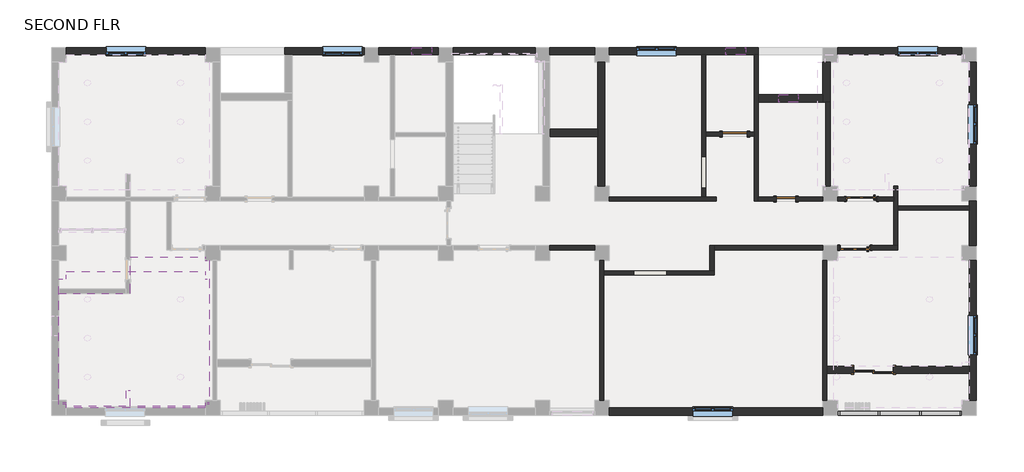
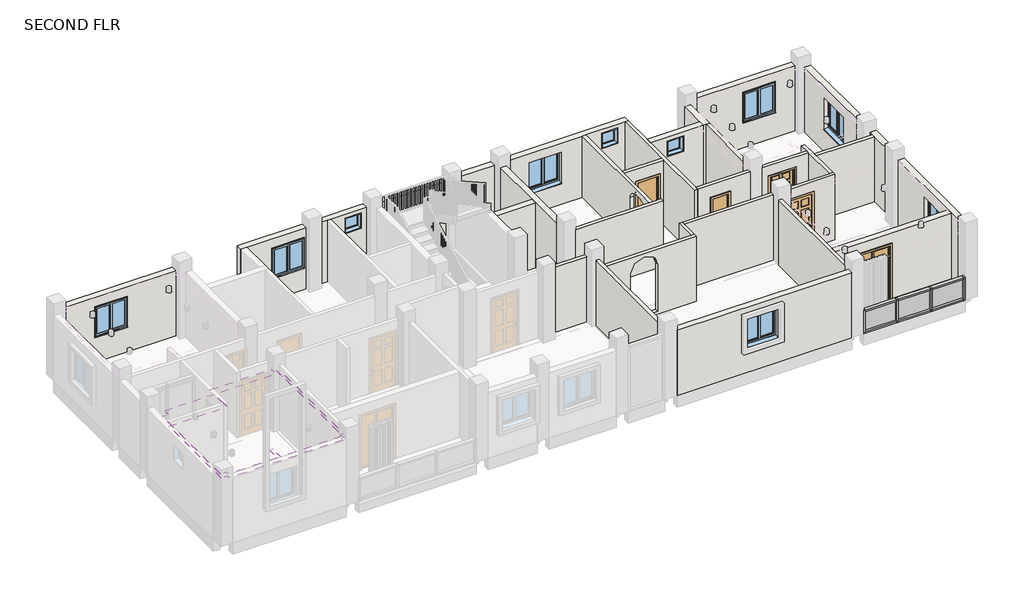
# One storey, part 2 of 5: 32 walls, 10 members, 10 windows, 5 doors, 3 plates, 2 coverings.
"""IFC4 building model written with IfcOpenShell, lengths in millimetres."""

from ifc_helpers import new_model, si_unit, point, frame, frame_2d, origin, place, context, project, spatial, polyline, circle_curve, ellipse_curve, trimmed, segment, composite_curve, outline, extrude, faceted_brep, transform, mapped, element, save
from ifc_brep_helpers import plane_surface, extruded_surface, advanced_brep
from components import door_double_sliding_4436dcad, door_c610b25b, door_03e3dfb5, single_flush_2_x_7_bath_room_door_025d1c86, door_1fe7f57d, member_5d96a33e, member_91edd790, member_410c6227, member_73c23c35, system_panel_glazed_2f542010, system_panel_glazed_876b4d55, window_80340324, w2_0001_4_x_4_window_9dec5fc7

model = new_model("IFC4")

# Units and contexts
model_context = context("Model", 3, world=origin())
ifc_project = project(units=[si_unit("LENGTHUNIT", "METRE", prefix="MILLI")], contexts=[model_context])

# Site, building, storey
site = spatial("IfcSite", under=ifc_project)
building = spatial("IfcBuilding", under=site)
storey = spatial("IfcBuildingStorey", under=building, Name="SECOND FLR", Elevation=6400.8)

# Coverings
placement = place(None, origin())
element("IfcCovering", 1, ObjectType="GWB on Mtl. Stud", at=placement, inside=storey, context=model_context, shape_type="SweptSolid", body=[
    extrude(outline(polyline([(-15145.3456086, -10773.5679047), (-15145.3456086, -7363.1659448), (-12959.7401855, -7363.1659448), (-12959.7401855, -6244.0794704), (-10649.5456086, -6244.0794704), (-10649.5456086, -6358.3794704), (-10535.2456086, -6358.3794704), (-10535.2456086, -6963.5679047), (-10535.2456086, -10773.5679047), (-10649.5456086, -10773.5679047), (-10649.5456086, -10887.8679047), (-12959.7401855, -10887.8679047), (-14916.7456086, -10887.8679047), (-14916.7456086, -10773.5679047), (-15145.3456086, -10773.5679047)]), holes=[polyline([(-14840.5456086, -10583.0679047), (-10840.0456086, -10583.0679047), (-10840.0456086, -6548.8794704), (-12654.9401855, -6548.8794704), (-12654.9401855, -7667.9659448), (-14840.5456086, -7667.9659448), (-14840.5456086, -10583.0679047)])]), frame((0.0, 0.0, 8839.2), z_axis=(0.0, 0.0, 1.0), x_axis=(1.0, 0.0, 0.0)), (0.0, 0.0, 1.0), 107.95),
    extrude(outline(polyline([(-14688.1456086, -10430.6679047), (-14688.1456086, -7820.3659448), (-12502.5401855, -7820.3659448), (-12502.5401855, -6701.2794704), (-10992.4456086, -6701.2794704), (-10992.4456086, -10430.6679047), (-14688.1456086, -10430.6679047)]), holes=[polyline([(-14535.7456086, -7972.7659448), (-14535.7456086, -10278.2679047), (-11144.8456086, -10278.2679047), (-11144.8456086, -6853.6794704), (-12350.1401855, -6853.6794704), (-12350.1401855, -7972.7659448), (-14535.7456086, -7972.7659448)])]), frame((0.0, 0.0, 8839.2), z_axis=(0.0, 0.0, 1.0), x_axis=(1.0, 0.0, 0.0)), (0.0, 0.0, 1.0), 107.95),
])
element("IfcCovering", 2, ObjectType="GWB on Mtl. Stud", at=placement, inside=storey, context=model_context, shape_type="SweptSolid", body=[
    extrude(outline(polyline([(-14916.7456086, -6917.1794704), (-14916.7456086, -6688.5794704), (-10649.5456086, -6688.5794704), (-10649.5456086, -6917.1794704), (-10535.2456086, -6917.1794704), (-10535.2456086, -10727.1794704), (-10649.5456086, -10727.1794704), (-10649.5456086, -10841.4794704), (-12959.7401855, -10841.4794704), (-12959.7401855, -10360.3659448), (-13086.7401855, -10360.3659448), (-13086.7401855, -10841.4794704), (-14916.7456086, -10841.4794704), (-14916.7456086, -10727.1794704), (-15145.3456086, -10727.1794704), (-15145.3456086, -6917.1794704), (-14916.7456086, -6917.1794704)]), holes=[composite_curve([segment(trimmed(circle_curve(frame_2d((-14269.0456086, -7552.1794704)), 76.2), [point((-14345.2456086, -7552.1794704))], [point((-14192.8456086, -7552.1794704))], True, "CARTESIAN"), True, "CONTINUOUS"), segment(trimmed(circle_curve(frame_2d((-14269.0456086, -7552.1794704)), 76.2), [point((-14192.8456086, -7552.1794704))], [point((-14345.2456086, -7552.1794704))], True, "CARTESIAN"), True, "CONTINUOUS")], self_intersect=False), composite_curve([segment(trimmed(circle_curve(frame_2d((-14269.0456086, -9939.7794704)), 76.2), [point((-14345.2456086, -9939.7794704))], [point((-14192.8456086, -9939.7794704))], True, "CARTESIAN"), True, "CONTINUOUS"), segment(trimmed(circle_curve(frame_2d((-14269.0456086, -9939.7794704)), 76.2), [point((-14192.8456086, -9939.7794704))], [point((-14345.2456086, -9939.7794704))], True, "CARTESIAN"), True, "CONTINUOUS")], self_intersect=False), composite_curve([segment(trimmed(circle_curve(frame_2d((-14269.0456086, -8745.9794704)), 76.2), [point((-14345.2456086, -8745.9794704))], [point((-14192.8456086, -8745.9794704))], True, "CARTESIAN"), True, "CONTINUOUS"), segment(trimmed(circle_curve(frame_2d((-14269.0456086, -8745.9794704)), 76.2), [point((-14192.8456086, -8745.9794704))], [point((-14345.2456086, -8745.9794704))], True, "CARTESIAN"), True, "CONTINUOUS")], self_intersect=False), composite_curve([segment(trimmed(circle_curve(frame_2d((-11411.5456086, -7552.1794704)), 76.2), [point((-11335.3456086, -7552.1794704))], [point((-11487.7456086, -7552.1794704))], True, "CARTESIAN"), True, "CONTINUOUS"), segment(trimmed(circle_curve(frame_2d((-11411.5456086, -7552.1794704)), 76.2), [point((-11487.7456086, -7552.1794704))], [point((-11335.3456086, -7552.1794704))], True, "CARTESIAN"), True, "CONTINUOUS")], self_intersect=False), composite_curve([segment(trimmed(circle_curve(frame_2d((-11411.5456086, -9939.7794704)), 76.2), [point((-11335.3456086, -9939.7794704))], [point((-11487.7456086, -9939.7794704))], True, "CARTESIAN"), True, "CONTINUOUS"), segment(trimmed(circle_curve(frame_2d((-11411.5456086, -9939.7794704)), 76.2), [point((-11487.7456086, -9939.7794704))], [point((-11335.3456086, -9939.7794704))], True, "CARTESIAN"), True, "CONTINUOUS")], self_intersect=False)]), frame((0.0, 0.0, 8966.2), z_axis=(0.0, 0.0, 1.0), x_axis=(1.0, 0.0, 0.0)), (0.0, 0.0, 1.0), 107.95),
])

# Doors
door_double_sliding_shape = door_double_sliding_4436dcad(model_context)
element("IfcDoor", 3, ObjectType="Door-Double-Sliding", at=placement, inside=storey, context=model_context, shape_type="MappedRepresentation", body=[
    mapped(door_double_sliding_shape, transform((9879.3128058, -9592.4679047, 6400.8), x_axis=(-1.0, 0.0, 0.0), y_axis=(0.0, -1.0, 0.0), z_axis=(0.0, 0.0, 1.0))),
])
door_shape = door_c610b25b(model_context)
element("IfcDoor", 4, ObjectType="Door-Interior-Single-6_Panel-Wood : 36\" x 84\"", at=placement, inside=storey, context=model_context, shape_type="MappedRepresentation", body=[
    mapped(door_shape, transform((9511.0128058, -4462.9044704, 6400.8), x_axis=(-1.0, 0.0, 0.0), y_axis=(0.0, -1.0, 0.0), z_axis=(0.0, 0.0, 1.0))),
])
door_2_shape = door_03e3dfb5(model_context)
element("IfcDoor", 5, ObjectType="Door-Interior-Single-6_Panel-Wood : 36\" x 84\"", at=placement, inside=storey, context=model_context, shape_type="MappedRepresentation", body=[
    mapped(door_2_shape, transform((9307.8128058, -5967.8544704, 6400.8), x_axis=(-1.0, 0.0, 0.0), y_axis=(0.0, -1.0, 0.0), z_axis=(0.0, 0.0, 1.0))),
])
single_flush_2_x_7_bath_room_door_shape = single_flush_2_x_7_bath_room_door_025d1c86(model_context)
element("IfcDoor", 6, ObjectType="Single-Flush : 2' X 7' BATH ROOM DOOR", at=placement, inside=storey, context=model_context, shape_type="MappedRepresentation", body=[
    mapped(single_flush_2_x_7_bath_room_door_shape, transform((7190.4916602, -4466.0794704, 6400.8), x_axis=(1.0, 0.0, 0.0), y_axis=(0.0, 1.0, 0.0), z_axis=(0.0, 0.0, 1.0))),
])
door_3_shape = door_1fe7f57d(model_context)
element("IfcDoor", 7, ObjectType="Single-Flush : 30\" x 80\"", at=placement, inside=storey, context=model_context, shape_type="MappedRepresentation", body=[
    mapped(door_3_shape, transform((5615.6916602, -2472.1794704, 6400.8), x_axis=(1.0, 0.0, 0.0), y_axis=(0.0, 1.0, 0.0), z_axis=(0.0, 0.0, 1.0))),
])

# Members
member_shape = member_5d96a33e(model_context)
element("IfcMember", 8, ObjectType="Rectangular Mullion : 2.5\" x 5\" rectangular", at=placement, inside=storey, context=model_context, shape_type="MappedRepresentation", body=[
    mapped(member_shape, transform((12520.9128058, -11052.9679047, 7315.2), x_axis=(0.0, 0.0, 1.0), y_axis=(0.0, -1.0, 0.0), z_axis=(1.0, 0.0, 0.0))),
])
element("IfcMember", 9, ObjectType="Rectangular Mullion : 2.5\" x 5\" rectangular", at=placement, inside=storey, context=model_context, shape_type="MappedRepresentation", body=[
    mapped(member_shape, transform((10012.6628059, -11052.9679047, 7315.2), x_axis=(0.0, 0.0, 1.0), y_axis=(0.0, -1.0, 0.0), z_axis=(1.0, 0.0, 0.0))),
])
element("IfcMember", 10, ObjectType="Rectangular Mullion : 2.5\" x 5\" rectangular", at=placement, inside=storey, context=model_context, shape_type="MappedRepresentation", body=[
    mapped(member_shape, transform((8837.9128058, -11052.9679047, 6400.8), x_axis=(0.0, 0.0, -1.0), y_axis=(0.0, -1.0, 0.0), z_axis=(-1.0, 0.0, 0.0))),
])
element("IfcMember", 11, ObjectType="Rectangular Mullion : 2.5\" x 5\" rectangular", at=placement, inside=storey, context=model_context, shape_type="MappedRepresentation", body=[
    mapped(member_shape, transform((11346.1628057, -11052.9679047, 6400.8), x_axis=(0.0, 0.0, -1.0), y_axis=(0.0, -1.0, 0.0), z_axis=(-1.0, 0.0, 0.0))),
])
member_2_shape = member_91edd790(model_context)
element("IfcMember", 12, ObjectType="Rectangular Mullion : 2.5\" x 5\" rectangular", at=placement, inside=storey, context=model_context, shape_type="MappedRepresentation", body=[
    mapped(member_2_shape, transform((11282.6628057, -11052.9679047, 7315.2), x_axis=(0.0, 0.0, 1.0), y_axis=(0.0, -1.0, 0.0), z_axis=(1.0, 0.0, 0.0))),
])
element("IfcMember", 13, ObjectType="Rectangular Mullion : 2.5\" x 5\" rectangular", at=placement, inside=storey, context=model_context, shape_type="MappedRepresentation", body=[
    mapped(member_2_shape, transform((10076.1628059, -11052.9679047, 6400.8), x_axis=(0.0, 0.0, -1.0), y_axis=(0.0, -1.0, 0.0), z_axis=(-1.0, 0.0, 0.0))),
])
member_3_shape = member_410c6227(model_context)
element("IfcMember", 14, ObjectType="Rectangular Mullion : 2.5\" x 5\" rectangular", at=placement, inside=storey, context=model_context, shape_type="MappedRepresentation", body=[
    mapped(member_3_shape, transform((10044.4128059, -11052.9679047, 6400.8), x_axis=(1.0, 0.0, 0.0), y_axis=(0.0, -1.0, 0.0), z_axis=(0.0, 0.0, -1.0))),
])
element("IfcMember", 15, ObjectType="Rectangular Mullion : 2.5\" x 5\" rectangular", at=placement, inside=storey, context=model_context, shape_type="MappedRepresentation", body=[
    mapped(member_3_shape, transform((11314.4128057, -11052.9679047, 6400.8), x_axis=(1.0, 0.0, 0.0), y_axis=(0.0, -1.0, 0.0), z_axis=(0.0, 0.0, -1.0))),
])
member_4_shape = member_73c23c35(model_context)
element("IfcMember", 16, ObjectType="Rectangular Mullion : 2.5\" x 5\" rectangular", at=placement, inside=storey, context=model_context, shape_type="MappedRepresentation", body=[
    mapped(member_4_shape, transform((12584.4128058, -11052.9679047, 6400.8), x_axis=(1.0, 0.0, 0.0), y_axis=(0.0, -1.0, 0.0), z_axis=(0.0, 0.0, -1.0))),
])
element("IfcMember", 17, ObjectType="Rectangular Mullion : 2.5\" x 5\" rectangular", at=placement, inside=storey, context=model_context, shape_type="MappedRepresentation", body=[
    mapped(member_4_shape, transform((8774.4128058, -11052.9679047, 7315.2), x_axis=(-1.0, 0.0, 0.0), y_axis=(0.0, -1.0, 0.0), z_axis=(0.0, 0.0, 1.0))),
])

# Plates
system_panel_glazed_shape = system_panel_glazed_2f542010(model_context)
element("IfcPlate", 18, ObjectType="System Panel : Glazed", at=placement, inside=storey, context=model_context, shape_type="MappedRepresentation", body=[
    mapped(system_panel_glazed_shape, transform((9425.2878058, -11052.9679047, 6464.3), x_axis=(1.0, 0.0, 0.0), y_axis=(0.0, 1.0, 0.0), z_axis=(0.0, 0.0, 1.0))),
])
element("IfcPlate", 19, ObjectType="System Panel : Glazed", at=placement, inside=storey, context=model_context, shape_type="MappedRepresentation", body=[
    mapped(system_panel_glazed_shape, transform((11933.5378057, -11052.9679047, 6464.3), x_axis=(1.0, 0.0, 0.0), y_axis=(0.0, 1.0, 0.0), z_axis=(0.0, 0.0, 1.0))),
])
system_panel_glazed_2_shape = system_panel_glazed_876b4d55(model_context)
element("IfcPlate", 20, ObjectType="System Panel : Glazed", at=placement, inside=storey, context=model_context, shape_type="MappedRepresentation", body=[
    mapped(system_panel_glazed_2_shape, transform((10679.4128058, -11052.9679047, 6464.3), x_axis=(1.0, 0.0, 0.0), y_axis=(0.0, 1.0, 0.0), z_axis=(0.0, 0.0, 1.0))),
])

# Walls
element("IfcWall", 21, ObjectType="EXTERIOR WALL 9\"", at=placement, inside=storey, context=model_context, shape_type="SweptSolid", body=[
    extrude(outline(polyline([(6400.8, 1767.5916602), (6400.8, 8317.2128058), (8991.6, 8317.2128058), (8991.6, 1767.5916602), (6400.8, 1767.5916602)]), holes=[polyline([(7400.8, 5552.1916602), (7400.8, 4332.9916602), (8620.0, 4332.9916602), (8620.0, 5552.1916602), (7400.8, 5552.1916602)])]), frame((0.0, -11116.4679047, 0.0), z_axis=(0.0, 1.0, 0.0), x_axis=(0.0, 0.0, 1.0)), (0.0, 0.0, 1.0), 228.6),
])
element("IfcWall", 22, ObjectType="EXTERIOR WALL 9\"", at=placement, inside=storey, context=model_context, shape_type="Brep", body=[
    faceted_brep([(13041.6128058, -10659.2679047, 6400.8), (13041.6128058, -6358.3794704, 6400.8), (13041.6128058, -6358.3794704, 8991.6), (13041.6128058, -10659.2679047, 8991.6), (13041.6128058, -9262.2679047, 7315.2), (13041.6128058, -9262.2679047, 8534.4), (13041.6128058, -8043.0679047, 8534.4), (13041.6128058, -8043.0679047, 7315.2), (12813.0128058, -10659.2679047, 6400.8), (12813.0128058, -10659.2679047, 8991.6), (12813.0128058, -9833.7679047, 8991.6), (12813.0128058, -9605.1679047, 8991.6), (12813.0128058, -6358.3794704, 8991.6), (12813.0128058, -6358.3794704, 6400.8), (12813.0128058, -9605.1679047, 6400.8), (12813.0128058, -9833.7679047, 6400.8), (12813.0128058, -9262.2679047, 7315.2), (12813.0128058, -8043.0679047, 7315.2), (12813.0128058, -8043.0679047, 8534.4), (12813.0128058, -9262.2679047, 8534.4)], [[[0, 1, 2, 3], [4, 5, 6, 7]], [[8, 9, 10, 11, 12, 13, 14, 15], [16, 17, 18, 19]], [[1, 0, 8, 15, 14, 13]], [[2, 1, 13, 12]], [[3, 2, 12, 11, 10, 9]], [[0, 3, 9, 8]], [[5, 4, 16, 19]], [[6, 5, 19, 18]], [[7, 6, 18, 17]], [[4, 7, 17, 16]]]),
])
element("IfcWall", 23, ObjectType="EXTERIOR WALL 9\"", at=placement, inside=storey, context=model_context, shape_type="Brep", body=[
    faceted_brep([(13041.6128058, -5901.1794704, 6400.8), (13041.6128058, -4529.5794704, 6400.8), (13041.6128058, -4529.5794704, 8991.6), (13041.6128058, -5901.1794704, 8991.6), (12813.0128058, -5901.1794704, 6400.8), (12813.0128058, -5901.1794704, 8991.6), (12813.0128058, -4808.9794704, 8991.6), (12813.0128058, -4681.9794704, 8991.6), (12813.0128058, -4529.5794704, 8991.6), (12813.0128058, -4529.5794704, 6400.8), (12813.0128058, -4681.9794704, 6400.8), (12813.0128058, -4808.9794704, 6400.8)], [[[0, 1, 2, 3]], [[4, 5, 6, 7, 8, 9, 10, 11]], [[1, 0, 4, 11, 10, 9]], [[2, 1, 9, 8]], [[3, 2, 8, 7, 6, 5]], [[0, 3, 5, 4]]]),
])
element("IfcWall", 24, ObjectType="EXTERIOR WALL 9\"", at=placement, inside=storey, context=model_context, shape_type="SweptSolid", body=[
    extrude(outline(polyline([(-4072.3794704, 6400.8), (-4072.3794704, 8991.6), (-262.3794704, 8991.6), (-262.3794704, 6400.8), (-4072.3794704, 6400.8)]), holes=[polyline([(-2776.9794704, 7315.2), (-1557.7794704, 7315.2), (-1557.7794704, 8534.4), (-2776.9794704, 8534.4), (-2776.9794704, 7315.2)])]), frame((12813.0128058, 0.0, 0.0), z_axis=(1.0, 0.0, 0.0), x_axis=(0.0, 1.0, 0.0)), (0.0, 0.0, 1.0), 228.6),
])
element("IfcWall", 25, ObjectType="EXTERIOR WALL 9\"", at=placement, inside=storey, context=model_context, shape_type="SweptSolid", body=[
    extrude(outline(polyline([(6400.8, 12584.4128058), (8991.6, 12584.4128058), (8991.6, 8774.4128058), (6400.8, 8774.4128058), (6400.8, 12584.4128058)]), holes=[polyline([(7400.8, 10628.6128058), (8620.0, 10628.6128058), (8620.0, 11847.8128058), (7400.8, 11847.8128058), (7400.8, 10628.6128058)])]), frame((0.0, -33.7794704, 0.0), z_axis=(0.0, 1.0, 0.0), x_axis=(0.0, 0.0, 1.0)), (0.0, 0.0, 1.0), 228.6),
])
element("IfcWall", 26, ObjectType="EXTERIOR WALL 9\"", at=placement, inside=storey, context=model_context, shape_type="SweptSolid", body=[
    extrude(outline(polyline([(6400.8, -14916.7456086), (6400.8, -10649.5456086), (8991.6, -10649.5456086), (8991.6, -14916.7456086), (6400.8, -14916.7456086)]), holes=[polyline([(7400.8, -13697.5456086), (8620.0, -13697.5456086), (8620.0, -12478.3456086), (7400.8, -12478.3456086), (7400.8, -13697.5456086)])]), frame((0.0, -33.7794704, 0.0), z_axis=(0.0, 1.0, 0.0), x_axis=(0.0, 0.0, 1.0)), (0.0, 0.0, 1.0), 228.6),
])
element("IfcWall", 27, ObjectType="EXTERIOR WALL 9\"", at=placement, inside=storey, context=model_context, shape_type="SweptSolid", body=[
    extrude(outline(polyline([(6400.8, 8444.2128058), (6400.8, 9269.7128058), (8534.4, 9269.7128058), (8534.4, 10488.9128058), (6400.8, 10488.9128058), (6400.8, 12813.0128058), (8991.6, 12813.0128058), (8991.6, 8444.2128058), (6400.8, 8444.2128058)])), frame((0.0, -9833.7679047, 0.0), z_axis=(0.0, 1.0, 0.0), x_axis=(0.0, 0.0, 1.0)), (0.0, 0.0, 1.0), 228.6),
])
element("IfcWall", 28, ObjectType="EXTERIOR WALL 9\"", at=placement, inside=storey, context=model_context, shape_type="Brep", body=[
    faceted_brep([(-5772.7456086, 194.8205296, 6400.8), (-8211.1456086, 194.8205296, 6400.8), (-8211.1456086, 194.8205296, 8991.6), (-5772.7456086, 194.8205296, 8991.6), (-7042.7456086, 194.8205296, 7400.8), (-5823.5456086, 194.8205296, 7400.8), (-5823.5456086, 194.8205296, 8620.0), (-7042.7456086, 194.8205296, 8620.0), (-5772.7456086, -33.7794704, 6400.8), (-5772.7456086, -33.7794704, 8991.6), (-7982.5456086, -33.7794704, 8991.6), (-8211.1456086, -33.7794704, 8991.6), (-8211.1456086, -33.7794704, 6400.8), (-7982.5456086, -33.7794704, 6400.8), (-7042.7456086, -33.7794704, 7400.8), (-7042.7456086, -33.7794704, 8620.0), (-5823.5456086, -33.7794704, 8620.0), (-5823.5456086, -33.7794704, 7400.8)], [[[0, 1, 2, 3], [4, 5, 6, 7]], [[8, 9, 10, 11, 12, 13], [14, 15, 16, 17]], [[1, 0, 8, 13, 12]], [[3, 2, 11, 10, 9]], [[0, 3, 9, 8]], [[2, 1, 12, 11]], [[15, 14, 4, 7]], [[16, 15, 7, 6]], [[17, 16, 6, 5]], [[14, 17, 5, 4]]]),
])
element("IfcWall", 29, ObjectType="EXTERIOR WALL 9\"", at=placement, inside=storey, context=model_context, shape_type="Brep", body=[
    faceted_brep([(-5315.5456086, -33.7794704, 6400.8), (-4959.9456086, -33.7794704, 6400.8), (-4832.9456086, -33.7794704, 6400.8), (-3486.7456086, -33.7794704, 6400.8), (-3486.7456086, -33.7794704, 8991.6), (-4832.9456086, -33.7794704, 8991.6), (-4959.9456086, -33.7794704, 8991.6), (-5315.5456086, -33.7794704, 8991.6), (-3689.9456086, -33.7794704, 8839.2), (-3689.9456086, -33.7794704, 8229.6), (-4299.5456086, -33.7794704, 8229.6), (-4299.5456086, -33.7794704, 8839.2), (-3486.7456086, 194.8205296, 6400.8), (-5315.5456086, 194.8205296, 6400.8), (-5315.5456086, 194.8205296, 8991.6), (-3486.7456086, 194.8205296, 8991.6), (-3689.9456086, 194.8205296, 8229.6), (-3689.9456086, 194.8205296, 8839.2), (-4299.5456086, 194.8205296, 8839.2), (-4299.5456086, 194.8205296, 8229.6)], [[[0, 1, 2, 3, 4, 5, 6, 7], [8, 9, 10, 11]], [[12, 13, 14, 15], [16, 17, 18, 19]], [[3, 2, 1, 0, 13, 12]], [[4, 3, 12, 15]], [[7, 6, 5, 4, 15, 14]], [[0, 7, 14, 13]], [[8, 17, 16, 9]], [[9, 16, 19, 10]], [[10, 19, 18, 11]], [[17, 8, 11, 18]]]),
])
element("IfcWall", 30, ObjectType="EXTERIOR WALL 9\"", at=placement, inside=storey, context=model_context, shape_type="SweptSolid", body=[
    extrude(outline(polyline([(-518.4083398, -33.7794704), (-3029.5456086, -33.7794704), (-3029.5456086, 194.8205296), (-518.4083398, 194.8205296), (-518.4083398, -33.7794704)])), frame((0.0, 0.0, 6400.8), z_axis=(0.0, 0.0, 1.0), x_axis=(1.0, 0.0, 0.0)), (0.0, 0.0, 1.0), 2590.8),
])
element("IfcWall", 31, ObjectType="EXTERIOR WALL 9\"", at=placement, inside=storey, context=model_context, shape_type="SweptSolid", body=[
    extrude(outline(polyline([(1310.3916602, -33.7794704), (-61.2083398, -33.7794704), (-61.2083398, 194.8205296), (1310.3916602, 194.8205296), (1310.3916602, -33.7794704)])), frame((0.0, 0.0, 6400.8), z_axis=(0.0, 0.0, 1.0), x_axis=(1.0, 0.0, 0.0)), (0.0, 0.0, 1.0), 2590.8),
])
element("IfcWall", 32, ObjectType="EXTERIOR WALL 9\"", at=placement, inside=storey, context=model_context, shape_type="Brep", body=[
    faceted_brep([(1767.5916602, -33.7794704, 6400.8), (4599.6916602, -33.7794704, 6400.8), (4726.6916602, -33.7794704, 6400.8), (6212.5916602, -33.7794704, 6400.8), (6339.5916602, -33.7794704, 6400.8), (6339.5916602, -33.7794704, 8991.6), (6212.5916602, -33.7794704, 8991.6), (4726.6916602, -33.7794704, 8991.6), (4599.6916602, -33.7794704, 8991.6), (1767.5916602, -33.7794704, 8991.6), (3824.9916602, -33.7794704, 8620.0), (3824.9916602, -33.7794704, 7400.8), (2605.7916602, -33.7794704, 7400.8), (2605.7916602, -33.7794704, 8620.0), (5945.8916602, -33.7794704, 8839.2), (5945.8916602, -33.7794704, 8229.6), (5336.2916602, -33.7794704, 8229.6), (5336.2916602, -33.7794704, 8839.2), (6339.5916602, 194.8205296, 6400.8), (1767.5916602, 194.8205296, 6400.8), (1767.5916602, 194.8205296, 8991.6), (6339.5916602, 194.8205296, 8991.6), (3824.9916602, 194.8205296, 7400.8), (3824.9916602, 194.8205296, 8620.0), (2605.7916602, 194.8205296, 8620.0), (2605.7916602, 194.8205296, 7400.8), (5945.8916602, 194.8205296, 8229.6), (5945.8916602, 194.8205296, 8839.2), (5336.2916602, 194.8205296, 8839.2), (5336.2916602, 194.8205296, 8229.6)], [[[0, 1, 2, 3, 4, 5, 6, 7, 8, 9], [10, 11, 12, 13], [14, 15, 16, 17]], [[18, 19, 20, 21], [22, 23, 24, 25], [26, 27, 28, 29]], [[4, 3, 2, 1, 0, 19, 18]], [[9, 8, 7, 6, 5, 21, 20]], [[0, 9, 20, 19]], [[5, 4, 18, 21]], [[23, 22, 11, 10]], [[24, 23, 10, 13]], [[25, 24, 13, 12]], [[22, 25, 12, 11]], [[14, 27, 26, 15]], [[15, 26, 29, 16]], [[16, 29, 28, 17]], [[27, 14, 17, 28]]]),
])
element("IfcWall", 33, ObjectType="EXTERIOR WALL 9\"", at=placement, inside=storey, context=model_context, shape_type="Brep", body=[
    faceted_brep([(8317.2128058, -262.3794704, 6400.8), (8317.2128058, -1252.9794704, 6400.8), (8317.2128058, -1481.5794704, 6400.8), (8317.2128058, -1481.5794704, 8991.6), (8317.2128058, -1252.9794704, 8991.6), (8317.2128058, -262.3794704, 8991.6), (8545.8128058, -262.3794704, 6400.8), (8545.8128058, -262.3794704, 8991.6), (8545.8128058, -1481.5794704, 8991.6), (8545.8128058, -1481.5794704, 6400.8), (8418.8128058, -1481.5794704, 6400.8), (8418.8128058, -1481.5794704, 8991.6)], [[[0, 1, 2, 3, 4, 5]], [[6, 7, 8, 9]], [[2, 1, 0, 6, 9, 10]], [[5, 4, 3, 11, 8, 7]], [[0, 5, 7, 6]], [[3, 2, 10, 9, 8, 11]]]),
])
element("IfcWall", 34, ObjectType="EXTERIOR WALL 9\"", at=placement, inside=storey, context=model_context, shape_type="SweptSolid", body=[
    extrude(outline(polyline([(6400.8, 6339.5916602), (6400.8, 8317.2128058), (8991.6, 8317.2128058), (8991.6, 6339.5916602), (6400.8, 6339.5916602)]), holes=[polyline([(8839.2, 7571.4916602), (8229.6, 7571.4916602), (8229.6, 6961.8916602), (8839.2, 6961.8916602), (8839.2, 7571.4916602)])]), frame((0.0, -1481.5794704, 0.0), z_axis=(0.0, 1.0, 0.0), x_axis=(0.0, 0.0, 1.0)), (0.0, 0.0, 1.0), 228.6),
])
element("IfcWall", 35, ObjectType="EXTERIOR WALL 9\"", at=placement, inside=storey, context=model_context, shape_type="Brep", body=[
    faceted_brep([(1399.2916602, -262.3794704, 6400.8), (1399.2916602, -2319.7794704, 6400.8), (1399.2916602, -2548.3794704, 6400.8), (1399.2916602, -4072.3794704, 6400.8), (1399.2916602, -4072.3794704, 8991.6), (1399.2916602, -2548.3794704, 8991.6), (1399.2916602, -2319.7794704, 8991.6), (1399.2916602, -262.3794704, 8991.6), (1627.8916602, -262.3794704, 6400.8), (1627.8916602, -262.3794704, 8991.6), (1627.8916602, -4072.3794704, 8991.6), (1627.8916602, -4072.3794704, 6400.8)], [[[0, 1, 2, 3, 4, 5, 6, 7]], [[8, 9, 10, 11]], [[3, 2, 1, 0, 8, 11]], [[4, 3, 11, 10]], [[7, 6, 5, 4, 10, 9]], [[0, 7, 9, 8]]]),
])
element("IfcWall", 36, ObjectType="EXTERIOR WALL 9\"", at=placement, inside=storey, context=model_context, shape_type="SweptSolid", body=[
    extrude(outline(polyline([(1399.2916602, -2548.3794704), (-61.2083398, -2548.3794704), (-61.2083398, -2319.7794704), (1399.2916602, -2319.7794704), (1399.2916602, -2548.3794704)])), frame((0.0, 0.0, 6400.8), z_axis=(0.0, 0.0, 1.0), x_axis=(1.0, 0.0, 0.0)), (0.0, 0.0, 1.0), 2590.8),
])
element("IfcWall", 37, ObjectType="INTERIOR WALL 5\"", at=placement, inside=storey, context=model_context, shape_type="Brep", body=[
    faceted_brep([(1589.7916602, -10659.2679047, 6400.8), (1589.7916602, -6802.8794704, 6400.8), (1589.7916602, -6675.8794704, 6400.8), (1589.7916602, -6358.3794704, 6400.8), (1589.7916602, -6358.3794704, 8991.6), (1589.7916602, -6675.8794704, 8991.6), (1589.7916602, -6802.8794704, 8991.6), (1589.7916602, -10659.2679047, 8991.6), (1462.7916602, -10659.2679047, 6400.8), (1462.7916602, -10659.2679047, 8991.6), (1462.7916602, -6358.3794704, 8991.6), (1462.7916602, -6358.3794704, 6400.8)], [[[0, 1, 2, 3, 4, 5, 6, 7]], [[8, 9, 10, 11]], [[3, 2, 1, 0, 8, 11]], [[4, 3, 11, 10]], [[7, 6, 5, 4, 10, 9]], [[0, 7, 9, 8]]]),
])
element("IfcWall", 38, ObjectType="INTERIOR WALL 5\"", at=placement, inside=storey, context=model_context, shape_type="Brep", body=[
    faceted_brep([(8444.2128058, -10659.2679047, 6400.8), (8444.2128058, -9833.7679047, 6400.8), (8444.2128058, -9605.1679047, 6400.8), (8444.2128058, -6358.3794704, 6400.8), (8444.2128058, -6358.3794704, 8991.6), (8444.2128058, -9605.1679047, 8991.6), (8444.2128058, -9833.7679047, 8991.6), (8444.2128058, -10659.2679047, 8991.6), (8317.2128058, -10659.2679047, 6400.8), (8317.2128058, -10659.2679047, 8991.6), (8317.2128058, -6358.3794704, 8991.6), (8317.2128058, -6358.3794704, 6400.8)], [[[0, 1, 2, 3, 4, 5, 6, 7]], [[8, 9, 10, 11]], [[3, 2, 1, 0, 8, 11]], [[4, 3, 11, 10]], [[7, 6, 5, 4, 10, 9]], [[0, 7, 9, 8]]]),
])
element("IfcWall", 39, ObjectType="INTERIOR WALL 5\"", at=placement, inside=storey, context=model_context, shape_type="SweptSolid", body=[
    extrude(outline(polyline([(10628.6128058, -4681.9794704), (12813.0128058, -4681.9794704), (12813.0128058, -4808.9794704), (10628.6128058, -4808.9794704), (10628.6128058, -4681.9794704)])), frame((0.0, 0.0, 6400.8), z_axis=(0.0, 0.0, 1.0), x_axis=(1.0, 0.0, 0.0)), (0.0, 0.0, 1.0), 2590.8),
])
element("IfcWall", 40, ObjectType="INTERIOR WALL 5\"", at=placement, inside=storey, context=model_context, shape_type="Brep", body=[
    faceted_brep([(10628.6128058, -6028.1794704, 8991.6), (8774.4128058, -6028.1794704, 8991.6), (8774.4128058, -6028.1794704, 6400.8), (8825.2128058, -6028.1794704, 6400.8), (8825.2128058, -6028.1794704, 8559.8), (9790.4128058, -6028.1794704, 8559.8), (9790.4128058, -6028.1794704, 6400.8), (10628.6128058, -6028.1794704, 6400.8), (8774.4128058, -5901.1794704, 8991.6), (10501.6128058, -5901.1794704, 8991.6), (10628.6128058, -5901.1794704, 8991.6), (10628.6128058, -5901.1794704, 6400.8), (10501.6128058, -5901.1794704, 6400.8), (9790.4128058, -5901.1794704, 6400.8), (9790.4128058, -5901.1794704, 8559.8), (8825.2128058, -5901.1794704, 8559.8), (8825.2128058, -5901.1794704, 6400.8), (8774.4128058, -5901.1794704, 6400.8)], [[[0, 1, 2, 3, 4, 5, 6, 7]], [[8, 9, 10, 11, 12, 13, 14, 15, 16, 17]], [[2, 17, 16, 3]], [[11, 7, 6, 13, 12]], [[1, 0, 10, 9, 8]], [[2, 1, 8, 17]], [[0, 7, 11, 10]], [[15, 4, 3, 16]], [[4, 15, 14, 5]], [[5, 14, 13, 6]]]),
])
element("IfcWall", 41, ObjectType="INTERIOR WALL 5\"", at=placement, inside=storey, context=model_context, shape_type="Brep", body=[
    faceted_brep([(10628.6128058, -5901.1794704, 6400.8), (10628.6128058, -4808.9794704, 6400.8), (10628.6128058, -4681.9794704, 6400.8), (10628.6128058, -4072.3794704, 6400.8), (10628.6128058, -4072.3794704, 8991.6), (10628.6128058, -4681.9794704, 8991.6), (10628.6128058, -4808.9794704, 8991.6), (10628.6128058, -5901.1794704, 8991.6), (10501.6128058, -5901.1794704, 6400.8), (10501.6128058, -5901.1794704, 8991.6), (10501.6128058, -4529.5794704, 8991.6), (10501.6128058, -4402.5794704, 8991.6), (10501.6128058, -4072.3794704, 8991.6), (10501.6128058, -4072.3794704, 6400.8), (10501.6128058, -4402.5794704, 6400.8), (10501.6128058, -4529.5794704, 6400.8)], [[[0, 1, 2, 3, 4, 5, 6, 7]], [[8, 9, 10, 11, 12, 13, 14, 15]], [[3, 2, 1, 0, 8, 15, 14, 13]], [[4, 3, 13, 12]], [[7, 6, 5, 4, 12, 11, 10, 9]], [[0, 7, 9, 8]]]),
])
element("IfcWall", 42, ObjectType="INTERIOR WALL 5\"", at=placement, inside=storey, context=model_context, shape_type="Brep", body=[
    faceted_brep([(6212.5916602, -33.7794704, 6400.8), (6212.5916602, -2408.6794704, 6400.8), (6212.5916602, -2535.6794704, 6400.8), (6212.5916602, -4529.5794704, 6400.8), (6212.5916602, -4529.5794704, 8991.6), (6212.5916602, -2535.6794704, 8991.6), (6212.5916602, -2408.6794704, 8991.6), (6212.5916602, -33.7794704, 8991.6), (6339.5916602, -33.7794704, 6400.8), (6339.5916602, -33.7794704, 8991.6), (6339.5916602, -1252.9794704, 8991.6), (6339.5916602, -1481.5794704, 8991.6), (6339.5916602, -4402.5794704, 8991.6), (6339.5916602, -4529.5794704, 8991.6), (6339.5916602, -4529.5794704, 6400.8), (6339.5916602, -4402.5794704, 6400.8), (6339.5916602, -1481.5794704, 6400.8), (6339.5916602, -1252.9794704, 6400.8)], [[[0, 1, 2, 3, 4, 5, 6, 7]], [[8, 9, 10, 11, 12, 13, 14, 15, 16, 17]], [[3, 2, 1, 0, 8, 17, 16, 15, 14]], [[7, 6, 5, 4, 13, 12, 11, 10, 9]], [[0, 7, 9, 8]], [[4, 3, 14, 13]]]),
])
element("IfcWall", 43, ObjectType="INTERIOR WALL 5\"", at=placement, inside=storey, context=model_context, shape_type="SweptSolid", body=[
    extrude(outline(polyline([(8418.8128058, -4072.3794704), (8418.8128058, -1481.5794704), (8545.8128058, -1481.5794704), (8545.8128058, -4072.3794704), (8418.8128058, -4072.3794704)])), frame((0.0, 0.0, 6400.8), z_axis=(0.0, 0.0, 1.0), x_axis=(1.0, 0.0, 0.0)), (0.0, 0.0, 1.0), 2590.8),
])
element("IfcWall", 44, ObjectType="INTERIOR WALL 5\"", at=placement, inside=storey, context=model_context, shape_type="Brep", body=[
    faceted_brep([(1767.5916602, -4529.5794704, 6400.8), (5044.1916602, -4529.5794704, 6400.8), (5044.1916602, -4529.5794704, 8991.6), (1767.5916602, -4529.5794704, 8991.6), (1767.5916602, -4402.5794704, 6400.8), (1767.5916602, -4402.5794704, 8991.6), (4599.6916602, -4402.5794704, 8991.6), (4726.6916602, -4402.5794704, 8991.6), (5044.1916602, -4402.5794704, 8991.6), (5044.1916602, -4402.5794704, 6400.8), (4726.6916602, -4402.5794704, 6400.8), (4599.6916602, -4402.5794704, 6400.8)], [[[0, 1, 2, 3]], [[4, 5, 6, 7, 8, 9, 10, 11]], [[1, 0, 4, 11, 10, 9]], [[2, 1, 9, 8]], [[3, 2, 8, 7, 6, 5]], [[0, 3, 5, 4]]]),
])
element("IfcWall", 45, ObjectType="INTERIOR WALL 5\"", at=placement, inside=storey, context=model_context, shape_type="AdvancedBrep", body=[
    advanced_brep(
    [(4599.6916602, -33.7794704, 6400.8), (4599.6916602, -4402.5794704, 6400.8), (4599.6916602, -4402.5794704, 8991.6), (4599.6916602, -33.7794704, 8991.6), (4599.6916602, -3162.9760679, 8459.4701015), (4599.6916602, -4128.1760679, 8459.4701015), (4599.6916602, -4128.1760679, 6579.8701015), (4599.6916602, -3162.9760679, 6579.8701015), (4726.6916602, -33.7794704, 6400.8), (4726.6916602, -33.7794704, 8991.6), (4726.6916602, -2408.6794704, 8991.6), (4726.6916602, -2535.6794704, 8991.6), (4726.6916602, -4402.5794704, 8991.6), (4726.6916602, -4402.5794704, 6400.8), (4726.6916602, -2535.6794704, 6400.8), (4726.6916602, -2408.6794704, 6400.8), (4726.6916602, -3162.9760679, 8459.4701015), (4726.6916602, -3162.9760679, 6579.8701015), (4726.6916602, -4128.1760679, 6579.8701015), (4726.6916602, -4128.1760679, 8459.4701015)],
    [
        (0, 1),
        (1, 2),
        (2, 3),
        (3, 0),
        (4, 5, ellipse_curve(frame((4599.6916602, -3645.5760679, 8459.4701015), z_axis=(1.0, 0.0, 0.0), x_axis=(0.0, -1.0, 0.0)), 482.6, 330.2)),
        (5, 6),
        (6, 7),
        (7, 4),
        (8, 9),
        (9, 10),
        (10, 11),
        (11, 12),
        (12, 13),
        (13, 14),
        (14, 15),
        (15, 8),
        (16, 17),
        (17, 18),
        (18, 19),
        (19, 16, ellipse_curve(frame((4726.6916602, -3645.5760679, 8459.4701015), z_axis=(-1.0, 0.0, 0.0), x_axis=(0.0, -1.0, 0.0)), 482.6, 330.2)),
        (3, 9),
        (8, 0),
        (1, 13),
        (12, 2),
        (4, 16),
        (19, 5),
        (18, 6),
        (17, 7),
    ],
    [
        plane_surface(frame((4599.6916602, 80.5205296, 6400.8), z_axis=(-1.0, 0.0, 0.0), x_axis=(0.0, -1.0, 0.0))),
        plane_surface(frame((4726.6916602, 80.5205296, 6400.8), z_axis=(1.0, 0.0, 0.0), x_axis=(0.0, 1.0, 0.0))),
        plane_surface(frame((1784.6412895, -33.7794704, 6400.8), z_axis=(0.0, 1.0, 0.0), x_axis=(1.0, 0.0, 0.0))),
        plane_surface(frame((1767.5916602, -4402.5794704, 6400.8), z_axis=(0.0, -1.0, 0.0), x_axis=(-1.0, 0.0, 0.0))),
        plane_surface(frame((4599.6916602, 80.5205296, 6400.8), z_axis=(0.0, 0.0, -1.0), x_axis=(1.0, 0.0, 0.0))),
        plane_surface(frame((4599.6916602, -4466.0794704, 8991.6), z_axis=(0.0, 0.0, 1.0), x_axis=(1.0, 0.0, 0.0))),
        extruded_surface(trimmed(ellipse_curve(frame((4790.1916602, -3645.5760679, 8459.4701015), z_axis=(1.0, 0.0, 0.0), x_axis=(0.0, -1.0, 0.0)), 482.6, 330.2), [point((4790.1916602, -3162.9760679, 8459.4701015))], [point((4790.1916602, -4128.1760679, 8459.4701015))], True, "CARTESIAN"), (-127.0, 0.0, 0.0), 127.0),
        plane_surface(frame((4599.6916602, -4128.1760679, 8459.4701015), z_axis=(0.0, 1.0, 0.0), x_axis=(1.0, 0.0, 0.0))),
        plane_surface(frame((4599.6916602, -4128.1760679, 6579.8701015), z_axis=(0.0, 0.0, 1.0), x_axis=(1.0, 0.0, 0.0))),
        plane_surface(frame((4599.6916602, -3162.9760679, 6579.8701015), z_axis=(0.0, -1.0, 0.0), x_axis=(1.0, 0.0, 0.0))),
    ],
    [
        (0, [[1, 2, 3, 4], [5, 6, 7, 8]]),
        (1, [[9, 10, 11, 12, 13, 14, 15, 16], [17, 18, 19, 20]]),
        (2, [[-4, 21, -9, 22]]),
        (3, [[-2, 23, -13, 24]]),
        (4, [[-1, -22, -16, -15, -14, -23]]),
        (5, [[-3, -24, -12, -11, -10, -21]]),
        (6, [[-5, 25, -20, 26]]),
        (7, [[-6, -26, -19, 27]]),
        (8, [[-7, -27, -18, 28]]),
        (9, [[-8, -28, -17, -25]]),
    ],
),
])
element("IfcWall", 46, ObjectType="INTERIOR WALL 5\"", at=placement, inside=storey, context=model_context, shape_type="SweptSolid", body=[
    extrude(outline(polyline([(8432.8, 5996.6916602), (6400.8, 5996.6916602), (6400.8, 6212.5916602), (8991.6, 6212.5916602), (8991.6, 4726.6916602), (6400.8, 4726.6916602), (6400.8, 5234.6916602), (8432.8, 5234.6916602), (8432.8, 5996.6916602)])), frame((0.0, -2535.6794704, 0.0), z_axis=(0.0, 1.0, 0.0), x_axis=(0.0, 0.0, 1.0)), (0.0, 0.0, 1.0), 127.0),
])
element("IfcWall", 47, ObjectType="INTERIOR WALL 5\"", at=placement, inside=storey, context=model_context, shape_type="SweptSolid", body=[
    extrude(outline(polyline([(8432.8, 7495.2916602), (6400.8, 7495.2916602), (6400.8, 8317.2128058), (8991.6, 8317.2128058), (8991.6, 6339.5916602), (6400.8, 6339.5916602), (6400.8, 6885.6916602), (8432.8, 6885.6916602), (8432.8, 7495.2916602)])), frame((0.0, -4529.5794704, 0.0), z_axis=(0.0, 1.0, 0.0), x_axis=(0.0, 0.0, 1.0)), (0.0, 0.0, 1.0), 127.0),
])
element("IfcWall", 48, ObjectType="INTERIOR WALL 5\"", at=placement, inside=storey, context=model_context, shape_type="SweptSolid", body=[
    extrude(outline(polyline([(8991.6, 10501.6128058), (8991.6, 8774.4128058), (6400.8, 8774.4128058), (6400.8, 9028.4128058), (8559.8, 9028.4128058), (8559.8, 9993.6128058), (6400.8, 9993.6128058), (6400.8, 10501.6128058), (8991.6, 10501.6128058)])), frame((0.0, -4529.5794704, 0.0), z_axis=(0.0, 1.0, 0.0), x_axis=(0.0, 0.0, 1.0)), (0.0, 0.0, 1.0), 127.0),
])
element("IfcWall", 49, ObjectType="INTERIOR WALL 5\"", at=placement, inside=storey, context=model_context, shape_type="SweptSolid", body=[
    extrude(outline(polyline([(-61.2083398, -5901.1794704), (1310.3916602, -5901.1794704), (1310.3916602, -6028.1794704), (-61.2083398, -6028.1794704), (-61.2083398, -5901.1794704)])), frame((0.0, 0.0, 6400.8), z_axis=(0.0, 0.0, 1.0), x_axis=(1.0, 0.0, 0.0)), (0.0, 0.0, 1.0), 2590.8),
])
element("IfcWall", 50, ObjectType="INTERIOR WALL 5\"", at=placement, inside=storey, context=model_context, shape_type="AdvancedBrep", body=[
    advanced_brep(
    [(1589.7916602, -6802.8794704, 6400.8), (4980.6916602, -6802.8794704, 6400.8), (4980.6916602, -6802.8794704, 8991.6), (1589.7916602, -6802.8794704, 8991.6), (2514.6258025, -6802.8794704, 8363.5597277), (3530.6258025, -6802.8794704, 8363.5597277), (3530.6258025, -6802.8794704, 6509.3597277), (2514.6258025, -6802.8794704, 6509.3597277), (1589.7916602, -6675.8794704, 6400.8), (1589.7916602, -6675.8794704, 8991.6), (4853.6916602, -6675.8794704, 8991.6), (4980.6916602, -6675.8794704, 8991.6), (4980.6916602, -6675.8794704, 6400.8), (4853.6916602, -6675.8794704, 6400.8), (2514.6258025, -6675.8794704, 8363.5597277), (2514.6258025, -6675.8794704, 6509.3597277), (3530.6258025, -6675.8794704, 6509.3597277), (3530.6258025, -6675.8794704, 8363.5597277)],
    [
        (0, 1),
        (1, 2),
        (2, 3),
        (3, 0),
        (4, 5, ellipse_curve(frame((3022.6258025, -6802.8794704, 8363.5597277), z_axis=(0.0, 1.0, 0.0), x_axis=(-1.0, 0.0, 0.0)), 508.0, 482.6)),
        (5, 6),
        (6, 7),
        (7, 4),
        (8, 9),
        (9, 10),
        (10, 11),
        (11, 12),
        (12, 13),
        (13, 8),
        (14, 15),
        (15, 16),
        (16, 17),
        (17, 14, ellipse_curve(frame((3022.6258025, -6675.8794704, 8363.5597277), z_axis=(0.0, -1.0, 0.0), x_axis=(-1.0, 0.0, 0.0)), 508.0, 482.6)),
        (3, 9),
        (8, 0),
        (1, 12),
        (11, 2),
        (4, 14),
        (17, 5),
        (16, 6),
        (15, 7),
    ],
    [
        plane_surface(frame((1526.2916602, -6802.8794704, 6400.8), z_axis=(0.0, -1.0, 0.0), x_axis=(1.0, 0.0, 0.0))),
        plane_surface(frame((1526.2916602, -6675.8794704, 6400.8), z_axis=(0.0, 1.0, 0.0), x_axis=(-1.0, 0.0, 0.0))),
        plane_surface(frame((1589.7916602, -10648.7570633, 6400.8), z_axis=(-1.0, 0.0, 0.0), x_axis=(0.0, 1.0, 0.0))),
        plane_surface(frame((4980.6916602, -6675.8794704, 6400.8), z_axis=(1.0, 0.0, 0.0), x_axis=(0.0, 1.0, 0.0))),
        plane_surface(frame((1526.2916602, -6802.8794704, 6400.8), z_axis=(0.0, 0.0, -1.0), x_axis=(0.0, 1.0, 0.0))),
        plane_surface(frame((4917.1916602, -6802.8794704, 8991.6), z_axis=(0.0, 0.0, 1.0), x_axis=(0.0, 1.0, 0.0))),
        extruded_surface(trimmed(ellipse_curve(frame((3022.6258025, -6612.3794704, 8363.5597277), z_axis=(0.0, 1.0, 0.0), x_axis=(-1.0, 0.0, 0.0)), 508.0, 482.6), [point((2514.6258025, -6612.3794704, 8363.5597277))], [point((3530.6258025, -6612.3794704, 8363.5597277))], True, "CARTESIAN"), (0.0, -127.0, 0.0), 127.0),
        plane_surface(frame((3530.6258025, -6802.8794704, 8363.5597277), z_axis=(-1.0, 0.0, 0.0), x_axis=(0.0, 1.0, 0.0))),
        plane_surface(frame((3530.6258025, -6802.8794704, 6509.3597277), z_axis=(0.0, 0.0, 1.0), x_axis=(0.0, 1.0, 0.0))),
        plane_surface(frame((2514.6258025, -6802.8794704, 6509.3597277), z_axis=(1.0, 0.0, 0.0), x_axis=(0.0, 1.0, 0.0))),
    ],
    [
        (0, [[1, 2, 3, 4], [5, 6, 7, 8]]),
        (1, [[9, 10, 11, 12, 13, 14], [15, 16, 17, 18]]),
        (2, [[-4, 19, -9, 20]]),
        (3, [[-2, 21, -12, 22]]),
        (4, [[-1, -20, -14, -13, -21]]),
        (5, [[-3, -22, -11, -10, -19]]),
        (6, [[-5, 23, -18, 24]]),
        (7, [[-6, -24, -17, 25]]),
        (8, [[-7, -25, -16, 26]]),
        (9, [[-8, -26, -15, -23]]),
    ],
),
])
element("IfcWall", 51, ObjectType="INTERIOR WALL 5\"", at=placement, inside=storey, context=model_context, shape_type="Brep", body=[
    faceted_brep([(4980.6916602, -6675.8794704, 6400.8), (4980.6916602, -6028.1794704, 6400.8), (4980.6916602, -5901.1794704, 6400.8), (4980.6916602, -5901.1794704, 8991.6), (4980.6916602, -6028.1794704, 8991.6), (4980.6916602, -6675.8794704, 8991.6), (4853.6916602, -6675.8794704, 6400.8), (4853.6916602, -6675.8794704, 8991.6), (4853.6916602, -5901.1794704, 8991.6), (4853.6916602, -5901.1794704, 6400.8)], [[[0, 1, 2, 3, 4, 5]], [[6, 7, 8, 9]], [[2, 1, 0, 6, 9]], [[5, 4, 3, 8, 7]], [[0, 5, 7, 6]], [[3, 2, 9, 8]]]),
])
element("IfcWall", 52, ObjectType="INTERIOR WALL 5\"", at=placement, inside=storey, context=model_context, shape_type="SweptSolid", body=[
    extrude(outline(polyline([(4980.6916602, -5901.1794704), (8317.2128058, -5901.1794704), (8317.2128058, -6028.1794704), (4980.6916602, -6028.1794704), (4980.6916602, -5901.1794704)])), frame((0.0, 0.0, 6400.8), z_axis=(0.0, 0.0, 1.0), x_axis=(1.0, 0.0, 0.0)), (0.0, 0.0, 1.0), 2590.8),
])

# Windows
window_shape = window_80340324(model_context)
element("IfcWindow", 53, ObjectType="Fixed : 24\" x 24\"", at=placement, inside=storey, context=model_context, shape_type="MappedRepresentation", body=[
    mapped(window_shape, transform((-3956.6456086, 80.5205296, 7315.2), x_axis=(1.0, 0.0, 0.0), y_axis=(0.0, 1.0, 0.0), z_axis=(0.0, 0.0, 1.0))),
])
element("IfcWindow", 54, ObjectType="Fixed : 24\" x 24\"", at=placement, inside=storey, context=model_context, shape_type="MappedRepresentation", body=[
    mapped(window_shape, transform((7304.7916602, -1367.2794704, 7315.2), x_axis=(1.0, 0.0, 0.0), y_axis=(0.0, 1.0, 0.0), z_axis=(0.0, 0.0, 1.0))),
])
element("IfcWindow", 55, ObjectType="Fixed : 24\" x 24\"", at=placement, inside=storey, context=model_context, shape_type="MappedRepresentation", body=[
    mapped(window_shape, transform((5679.1916602, 80.5205296, 7315.2), x_axis=(1.0, 0.0, 0.0), y_axis=(0.0, 1.0, 0.0), z_axis=(0.0, 0.0, 1.0))),
])
w2_0001_4_x_4_window_shape = w2_0001_4_x_4_window_9dec5fc7(model_context)
element("IfcWindow", 56, ObjectType="w2.0001 : 4' X 4' WINDOW", at=placement, inside=storey, context=model_context, shape_type="MappedRepresentation", body=[
    mapped(w2_0001_4_x_4_window_shape, transform((4942.5916602, -11002.1679047, 6400.8), x_axis=(-1.0, 0.0, 0.0), y_axis=(0.0, -1.0, 0.0), z_axis=(0.0, 0.0, 1.0))),
])
element("IfcWindow", 57, ObjectType="w2.0001 : 4' X 4' WINDOW", at=placement, inside=storey, context=model_context, shape_type="MappedRepresentation", body=[
    mapped(w2_0001_4_x_4_window_shape, transform((11238.2128058, 80.5205296, 6400.8), x_axis=(1.0, 0.0, 0.0), y_axis=(0.0, 1.0, 0.0), z_axis=(0.0, 0.0, 1.0))),
])
element("IfcWindow", 58, ObjectType="w2.0001 : 4' X 4' WINDOW", at=placement, inside=storey, context=model_context, shape_type="MappedRepresentation", body=[
    mapped(w2_0001_4_x_4_window_shape, transform((3215.3916602, 80.5205296, 6400.8), x_axis=(-1.0, 0.0, 0.0), y_axis=(0.0, -1.0, 0.0), z_axis=(0.0, 0.0, 1.0))),
])
element("IfcWindow", 59, ObjectType="w2.0001 : 4' X 4' WINDOW", at=placement, inside=storey, context=model_context, shape_type="MappedRepresentation", body=[
    mapped(w2_0001_4_x_4_window_shape, transform((-6433.1456086, 80.5205296, 6400.8), x_axis=(1.0, 0.0, 0.0), y_axis=(0.0, 1.0, 0.0), z_axis=(0.0, 0.0, 1.0))),
])
element("IfcWindow", 60, ObjectType="w2.0001 : 4' X 4' WINDOW", at=placement, inside=storey, context=model_context, shape_type="MappedRepresentation", body=[
    mapped(w2_0001_4_x_4_window_shape, transform((-13087.9456086, 80.5205296, 6400.8), x_axis=(1.0, 0.0, 0.0), y_axis=(0.0, 1.0, 0.0), z_axis=(0.0, 0.0, 1.0))),
])
element("IfcWindow", 61, ObjectType="w2.0001 : 4' X 4' WINDOW", at=placement, inside=storey, context=model_context, shape_type="MappedRepresentation", body=[
    mapped(w2_0001_4_x_4_window_shape, transform((12927.3128058, -8652.6679047, 6315.2), x_axis=(0.0, 1.0, 0.0), y_axis=(-1.0, 0.0, 0.0), z_axis=(0.0, 0.0, 1.0))),
])
element("IfcWindow", 62, ObjectType="w2.0001 : 4' X 4' WINDOW", at=placement, inside=storey, context=model_context, shape_type="MappedRepresentation", body=[
    mapped(w2_0001_4_x_4_window_shape, transform((12927.3128058, -2167.3794704, 6315.2), x_axis=(0.0, 1.0, 0.0), y_axis=(-1.0, 0.0, 0.0), z_axis=(0.0, 0.0, 1.0))),
])

save(model, "model.ifc")

# Revit data of these elements
# Type "GWB on Mtl. Stud"
#   Assembly Code = "C3030220"
#   built-in parameter 1002203 = 1 (stored number, unit not read)
#   built-in parameter 1002202 = 1 (stored number, unit not read)
#   Layers, outside or top first: 0' - 3 5/8" "WHITE CEILING 6\"" (function 1); 0' - 0 5/8" "WHITE CEILING 6\"" (function 5)
# Type "Door-Double-Sliding"
#   Type Mark = "14"
#   Construction Type Id = "opn-d45"
#   Assembly Code = "C1020"
#   Analytic Construction = "Wood frame, double glass door "
#   Thickness = 0' - 2"
#   Thermal Resistance (R) = 1.8150 (h·ft²·°F)/BTU
#   Heat Transfer Coefficient (U) = 0.5510 BTU/(h·ft²·°F)
#   Height = 7' - 0"
#   Rail Width = 0' - 2"
#   Stiles = 0' - 2"
#   Trim Projection Ext = 0' - 1"
#   Trim Projection Int = 0' - 1"
#   Trim Width = 0' - 3"
#   Width = 4' - 0"
#   Define Thermal Properties by = 1
#   Glazing = Glass
#   Panel Material = Wood - Birch - Solid Stained Light Low Gloss
#   Trim Material = Paint - Sienna
#   Visual Light Transmittance = 0
#   Solar Heat Gain Coefficient = 0
#   Function = (empty or 0)
#   Wall Closure = (empty or 0)
# Type "Door-Interior-Single-6_Panel-Wood : 36\" x 84\""
#   Type Mark = "10"
#   Assembly Code = "C1020300"
#   Analytic Construction = "Wooden"
#   Top Rail = 0' - 4 11/16"
#   Top Panel = 0' - 11"
#   Thickness = 0' - 1 3/8"
#   Thermal Resistance (R) = 2.5876 (h·ft²·°F)/BTU
#   Swing Angle [instance default] = 90.00°
#   Stiles = 0' - 4 3/4"
#   Rough Width = 3' - 2"
#   Rough Height = 7' - 1"
#   Mullion = 0' - 4 1/2"
#   Lock Rail = 0' - 7 1/2"
#   Intermediate Rail = 0' - 4 1/2"
#   Height = 7' - 0"
#   Width = 3' - 0"
#   Heat Transfer Coefficient (U) = 0.3865 BTU/(h·ft²·°F)
#   Bottom Rail = 0' - 9 1/8"
#   Trim Material = Cherry
#   Panel Material = Cherry
#   Frame Material = Cherry
#   Door Handle Material = Aluminum
#   Visual Light Transmittance = 0
#   Solar Heat Gain Coefficient = 0
#   Wall Closure = (empty or 0)
#   Function = (empty or 0)
# Type "Single-Flush : 2' X 7' BATH ROOM DOOR"
#   Type Mark = "11"
#   Construction Type Id = "MDOOR"
#   Assembly Code = "C1020"
#   Analytic Construction = "Metal"
#   Thickness = 0' - 2"
#   Heat Transfer Coefficient (U) = 0.651978 BTU/(h·ft²·°F)
#   Height = 6' - 8"
#   Trim Projection Ext = 0' - 1"
#   Trim Projection Int = 0' - 1"
#   Trim Width = 0' - 3"
#   Width = 2' - 0"
#   Define Thermal Properties by = 1
#   Door Material = Door - Panel
#   Frame Material = Door - Frame
#   Visual Light Transmittance = 0
#   Solar Heat Gain Coefficient = 0
#   Function = (empty or 0)
#   Wall Closure = (empty or 0)
# Type "Single-Flush : 30\" x 80\""
#   Type Mark = "5"
#   Construction Type Id = "MDOOR"
#   Assembly Code = "C1020"
#   Analytic Construction = "Metal"
#   Thickness = 0' - 2"
#   Heat Transfer Coefficient (U) = 0.651978 BTU/(h·ft²·°F)
#   Height = 6' - 8"
#   Trim Projection Ext = 0' - 1"
#   Trim Projection Int = 0' - 1"
#   Trim Width = 0' - 3"
#   Width = 2' - 6"
#   Define Thermal Properties by = 1
#   Define Thermal Properties by = 1
#   Door Material = Door - Panel
#   Frame Material = Door - Frame
#   Visual Light Transmittance = 0
#   Solar Heat Gain Coefficient = 0
#   Function = (empty or 0)
#   Wall Closure = (empty or 0)
# Type "Rectangular Mullion : 2.5\" x 5\" rectangular"
#   built-in parameter 1007304 = 0.416667 (stored number, unit not read)
#   built-in parameter 1007301 = 0.104167 (stored number, unit not read)
#   built-in parameter 1007300 = 0.104167 (stored number, unit not read)
# Type "System Panel : Glazed"
#   Construction Type Id = "GSP4R"
#   Analytic Construction = "1/8 in Pilkington single glazing"
#   Visual Light Transmittance = 0.9
#   Solar Heat Gain Coefficient = 0.86
#   Heat Transfer Coefficient (U) = 1.18115 BTU/(h·ft²·°F)
#   Define Thermal Properties by = 1
# Type "EXTERIOR WALL 9\""
#   Assembly Code = "B2010"
#   Layers, outside or top first: 0' - 9" "SAND BEIGE PAINT" (function 1)
# Type "INTERIOR WALL 5\""
#   Assembly Code = "B2010"
#   Layers, outside or top first: 0' - 5" "SAND BEIGE PAINT" (function 1)
# Type "Fixed : 24\" x 24\""
#   Type Mark = "3"
#   Construction Type Id = "GSP4R"
#   Assembly Code = "B2020100"
#   Analytic Construction = "1/8 in Pilkington single glazing"
#   Visual Light Transmittance = 0.9
#   Solar Heat Gain Coefficient = 0.78
#   Heat Transfer Coefficient (U) = 0.6496 BTU/(h·ft²·°F)
#   Height = 2' - 0"
#   Default Sill Height = 3' - 0"
#   Width = 2' - 0"
#   Window Inset = 0' - 0 3/4"
#   Define Thermal Properties by = 1
#   Define Thermal Properties by = 1
#   Glass Pane Material = Glass
#   Sash Material = Sash
#   Wall Closure = (empty or 0)
# Type "w2.0001 : 4' X 4' WINDOW"
#   Type Mark = "21"
#   Operation = "DoublePanelVertical"
#   Keynote = "16.05.01"
#   Analytic Construction = "<None>"
#   Rough Width = 4' - 0"
#   Rough Height = 4' - 0"
#   Rahmentiefe = 0' - 2.3622"
#   Rahmenhöhe unten = 0' - 3.14961"
#   Rahmehöhe oben = 0' - 3.14961"
#   Rahmenbreite = 0' - 2.3622"
#   Height = 4' - 0"
#   Flügeltiefe = 0' - 2.3622"
#   Flügelbreite = 0' - 2.3622"
#   Einbautiefe (von außen) [instance default] = 0' - 5.51181"
#   Width = 4' - 0"
#   Kippflügel [instance default] = yes
#   Drehflügel im Grundriß darstellen [instance default] = no
#   Drehflügel [instance default] = yes
#   Define Thermal Properties by = 1
#   Rahmen [instance default] = none
#   Glas [instance default] = none
#   Flügel [instance default] = none
#   Fensterbank aussen [instance default] = none
#   Fensterbank innen [instance default] = none
#   Wall Closure = (empty or 0)
# Element 1 (IfcCovering, "GWB on Mtl. Stud")
#   Height Offset From Level = 8' - 0"
#   Phase Created = New Construction
#   Materials on its faces: "WHITE CEILING 6\""
# Element 2 (IfcCovering, "GWB on Mtl. Stud")
#   Height Offset From Level = 8' - 5"
#   Phase Created = New Construction
#   Materials on its faces: "WHITE CEILING 6\""
# Element 3 (IfcDoor, "Door-Double-Sliding")
#   Phase Created = New Construction
#   Materials on its faces: "Paint - Sienna", "Wood - Birch - Solid Stained Light Low Gloss", "Glass"
# Elements 4, 5 (IfcDoor, "Door-Interior-Single-6_Panel-Wood : 36\" x 84\"")
#   Swing Angle = 90.00°
#   Phase Created = New Construction
#   Materials on its faces: "Cherry", "Aluminum"
# Element 6 (IfcDoor, "Single-Flush : 2' X 7' BATH ROOM DOOR")
#   Phase Created = New Construction
#   Materials on its faces: "Door - Frame", "Door - Panel"
# Element 7 (IfcDoor, "Single-Flush : 30\" x 80\"")
#   Phase Created = New Construction
#   Materials on its faces: "Door - Frame", "Door - Panel"
# Elements 8, 9, 10, 11, 12, 13, 14, 15, 16, 17 (IfcMember, "Rectangular Mullion : 2.5\" x 5\" rectangular")
#   Phase Created = New Construction
#   Materials on its faces: "WINDOW FRAMING"
# Elements 18, 19, 20 (IfcPlate, "System Panel : Glazed")
#   Phase Created = New Construction
#   Materials on its faces: "Glass"
# Elements 21, 22, 23, 24, 25, 26, 27, 28, 29, 30, 31, 32, 33, 34, 35, 36 (IfcWall, "EXTERIOR WALL 9\"")
#   Top Offset = 8' - 6"
#   Base Offset = 0' - 0"
#   wall height = 8' - 6"
#   Phase Created = New Construction
#   Base Constraint = SECOND FLR
#   Top Constraint = SECOND FLR
#   Materials on its faces: "SAND BEIGE PAINT"
# Elements 37, 38, 39, 40, 41, 42, 43, 44, 45, 46, 47, 48, 49, 50, 51, 52 (IfcWall, "INTERIOR WALL 5\"")
#   Top Offset = 8' - 6"
#   Base Offset = 0' - 0"
#   wall height = 8' - 6"
#   Phase Created = New Construction
#   Base Constraint = SECOND FLR
#   Top Constraint = SECOND FLR
#   Materials on its faces: "SAND BEIGE PAINT"
# Element 53 (IfcWindow, "Fixed : 24\" x 24\"")
#   Mark = "81"
#   Phase Created = New Construction
#   Materials on its faces: "Sash", "Glass"
# Element 54 (IfcWindow, "Fixed : 24\" x 24\"")
#   Mark = "82"
#   Phase Created = New Construction
#   Materials on its faces: "Sash", "Glass"
# Element 55 (IfcWindow, "Fixed : 24\" x 24\"")
#   Mark = "83"
#   Phase Created = New Construction
#   Materials on its faces: "Sash", "Glass"
# Element 56 (IfcWindow, "w2.0001 : 4' X 4' WINDOW")
#   Mark = "75"
#   Einbautiefe (von außen) = 0' - 5.51181"
#   Kippflügel = yes
#   Drehflügel im Grundriß darstellen = no
#   Drehflügel = yes
#   Rahmen = none
#   Glas = none
#   Flügel = none
#   Fensterbank innen = none
#   Fensterbank aussen = none
#   Phase Created = New Construction
#   Materials on its faces: "Fenster - Kunststoff", "Fenster - Kunststoff weiss", "Glass", "Fenster - Holz"
# Element 57 (IfcWindow, "w2.0001 : 4' X 4' WINDOW")
#   Mark = "77"
#   Einbautiefe (von außen) = 0' - 5.51181"
#   Kippflügel = yes
#   Drehflügel im Grundriß darstellen = no
#   Drehflügel = yes
#   Rahmen = none
#   Glas = none
#   Flügel = none
#   Fensterbank innen = none
#   Fensterbank aussen = none
#   Phase Created = New Construction
#   Materials on its faces: "Fenster - Kunststoff", "Fenster - Kunststoff weiss", "Glass", "Fenster - Holz"
# Element 58 (IfcWindow, "w2.0001 : 4' X 4' WINDOW")
#   Mark = "78"
#   Einbautiefe (von außen) = 0' - 5.51181"
#   Kippflügel = yes
#   Drehflügel im Grundriß darstellen = no
#   Drehflügel = yes
#   Rahmen = none
#   Glas = none
#   Flügel = none
#   Fensterbank innen = none
#   Fensterbank aussen = none
#   Phase Created = New Construction
#   Materials on its faces: "Fenster - Kunststoff", "Fenster - Kunststoff weiss", "Glass", "Fenster - Holz"
# Element 59 (IfcWindow, "w2.0001 : 4' X 4' WINDOW")
#   Mark = "79"
#   Einbautiefe (von außen) = 0' - 5.51181"
#   Kippflügel = yes
#   Drehflügel im Grundriß darstellen = no
#   Drehflügel = yes
#   Rahmen = none
#   Glas = none
#   Flügel = none
#   Fensterbank innen = none
#   Fensterbank aussen = none
#   Phase Created = New Construction
#   Materials on its faces: "Fenster - Kunststoff", "Fenster - Kunststoff weiss", "Glass", "Fenster - Holz"
# Element 60 (IfcWindow, "w2.0001 : 4' X 4' WINDOW")
#   Mark = "80"
#   Einbautiefe (von außen) = 0' - 5.51181"
#   Kippflügel = yes
#   Drehflügel im Grundriß darstellen = no
#   Drehflügel = yes
#   Rahmen = none
#   Glas = none
#   Flügel = none
#   Fensterbank innen = none
#   Fensterbank aussen = none
#   Phase Created = New Construction
